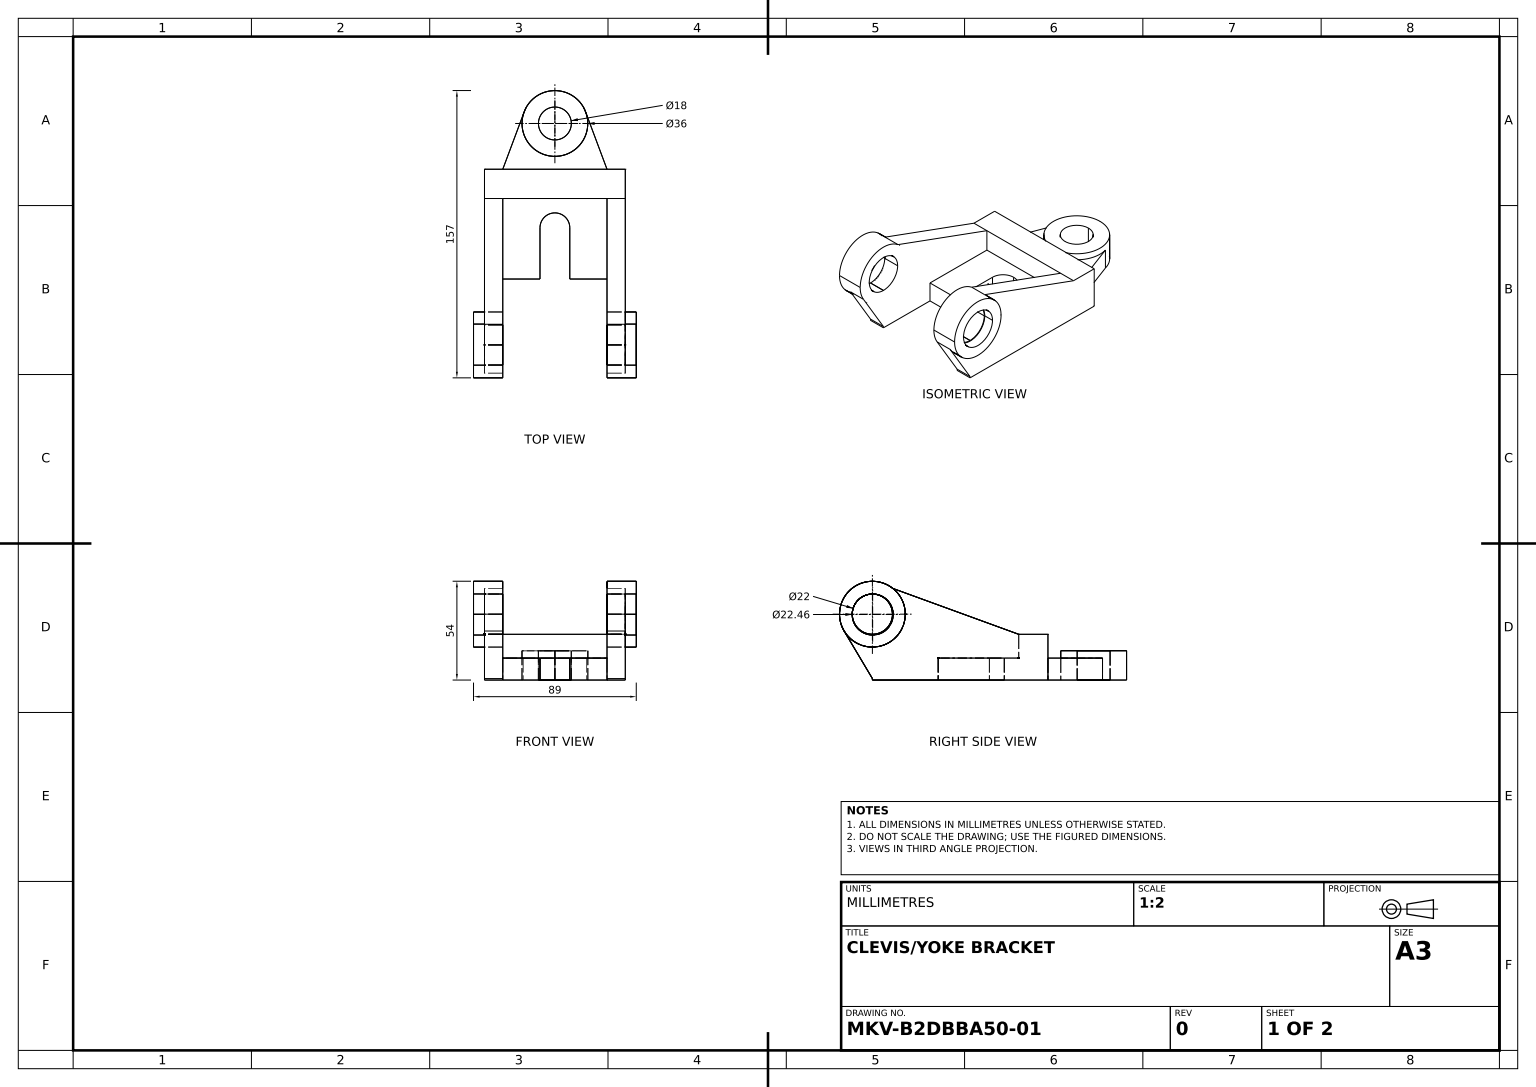
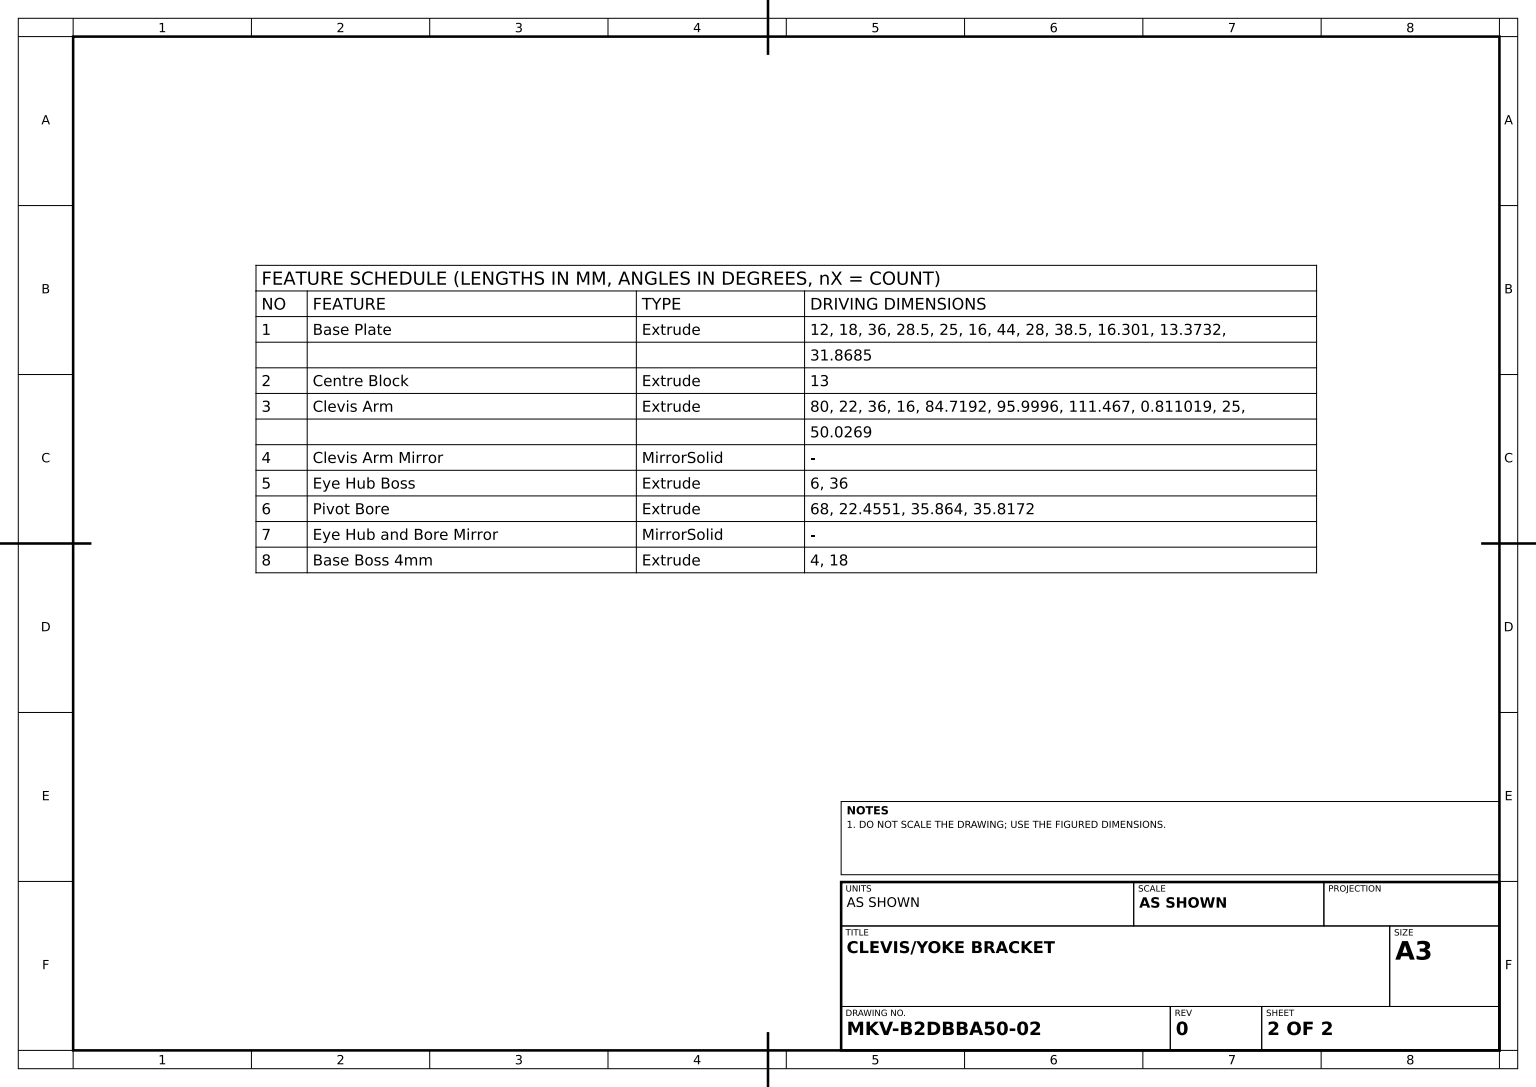
SolidWorks part; units mm, degrees
material "Plain Carbon Steel"
ref_plane "Front Plane" through (0, 0, 0) normal (0, 0, 1) x (1, 0, 0)
ref_plane "Top Plane" through (0, 0, 0) normal (0, 1, 0) x (1, 0, 0)
ref_plane "Right Plane" through (0, 0, 0) normal (1, 0, 0) x (0, 0, -1)
sketch "Base Plate Sketch" plane through (0, 0, 0) normal (0, 1, 0) x (1, 0, 0)
  line L0 (0, -13.3732) -> (-28.5, -13.3732)
  line L1 (-28.5, -13.3732) -> (28.5, -13.3732)
  line L2 (-28.5, -13.3732) -> (-17.3347, 16.4754)
  line L3 (17.3347, 16.4754) -> (28.5, -13.3732)
  line L4 (-8.1505, -45.3732) -> (-8.1505, -73.3732)
  line L5 (-28.5, -13.3732) -> (28.5, -13.3732)
  line L7 (-28.5, -29.3732) -> (28.5, -29.3732)
  line L9 (-28.5, -29.3732) -> (28.5, -29.3732)
  line L10 (-28.5, -29.3732) -> (-28.5, -73.3732)
  line L11 (-28.5, -73.3732) -> (-8.1505, -73.3732)
  line L12 (28.5, -29.3732) -> (28.5, -73.3732)
  line L13 (8.1505, -45.3732) -> (8.1505, -73.3732)
  line L14 (8.1505, -73.3732) -> (28.5, -73.3732)
  line L16 (-38.5, -13.3732) -> (38.5, -13.3732)
  line L17 (-38.5, -13.3732) -> (-38.5, -29.3732)
  line L18 (-38.5, -29.3732) -> (38.5, -29.3732)
  line L19 (38.5, -13.3732) -> (38.5, -29.3732)
  circle A0 centre (0, 11.6268) radius 9
  circle A1 centre (0, 11.6268) radius 18
  arc A2 (8.1505, -45.3732) -> (-8.1505, -45.3732) centre (0, -45.3732) ccw
  point P15 (0, -29.3732)
  dimension "D1" = 18
  dimension "D2" = 36
  dimension "D3" = 28.5
  dimension "D4" = 0
  dimension "D5" = 28.5
  dimension "D6" = 25
  dimension "D7" = 16
  dimension "D8" = 28.5
  dimension "D9" = 28.5
  dimension "D10" = 44
  dimension "D11" = 28
  dimension "D12" = 38.5
  dimension "D13" = 38.5
  dimension "D14" = 16.301
  dimension "D15" = 13.3732
  dimension "D16" = 31.8685
extrude "Base Plate" add sketch "Base Plate Sketch" along normal blind 12 contours A2 L13 L14 L12 L7 L10 L11 L4 | L19 L16 L1 L0 L17 L18 L7 | A1 L2 L0 L1 L3 | A1 A0
sketch "Centre Block Sketch" plane through (0, 12, 0) normal (0, 1, 0) x (1, 0, 0)
  line L1 (-38.5, -13.3732) -> (38.5, -13.3732)
  line L2 (-38.5, -13.3732) -> (-38.5, -29.3732)
  line L3 (-38.5, -29.3732) -> (38.5, -29.3732)
  line L4 (38.5, -13.3732) -> (38.5, -29.3732)
extrude "Centre Block" add sketch "Centre Block Sketch" along normal blind 13
sketch "Arm Reference Sketch" plane through (0, 0, 29.3732) normal (0, 0, 1) x (1, 0, 0)
  line L1 (38.5, 25) -> (28.5, 25)
  line L2 (38.5, 25) -> (38.5, 0)
  line L3 (38.5, 0) -> (28.5, 0)
  line L4 (28.5, 25) -> (28.5, 0)
  line L5 (-28.5, 0) -> (-38.5, 0)
  line L6 (-28.5, 0) -> (-28.5, 25)
  line L7 (-28.5, 25) -> (-38.5, 25)
  line L8 (-38.5, 0) -> (-38.5, 25)
sketch "Clevis Arm Sketch" plane through (38.5, 0, 0) normal (1, 0, 0) x (0, 0, -1)
  line L0 (-29.3732, 25) -> (-98.0924, 50.0269)
  line L1 (-29.3732, 0) -> (-109.3732, 0)
  line L2 (-29.3732, 0) -> (-29.3732, 25)
  line L3 (-109.3728, 25) -> (-109.3732, 25)
  line L4 (-109.3732, 0) -> (-109.3732, 0.811)
  line L5 (-109.3732, 0.811) -> (-124.8397, 26.7928)
  line L6 (-13.3732, 0) -> (-29.3732, 0) construction
  line L7 (-13.3732, 25) -> (-13.3732, 0) construction
  circle A0 centre (-109.3728, 36) radius 11
  circle A1 centre (-109.3728, 36) radius 18
  line M5 (-29.3732, 25) -> (-29.3732, 0)
  dimension "D2" = 22
  dimension "D3" = 36
  dimension "D1" = 80
  dimension "D4" = 36
  dimension "D5" = 16
  dimension "D6" = 84.7192
  dimension "D7" = 95.9996
  dimension "D8" = 111.4665
  dimension "D9" = 0.811
  dimension "D10" = 25
  dimension "D11" = 50.0269
extrude "Clevis Arm" add sketch "Clevis Arm Sketch" against normal up to vertex (10 mm away) contours A1 L5 L4 L1 L0 M5 | A1 A0 L3 up to point (28.5, 25, 29.3732)
mirror "Clevis Arm Mirror" about plane through (0, 0, 0) normal (1, 0, 0) of bodies 107
sketch "Eye Hub Sketch" plane through (38.5, 0, 0) normal (1, 0, 0) x (0, 0, -1)
  circle A0 centre (-109.3728, 36) radius 18
  dimension "D1" = 36
extrude "Eye Hub Boss" add sketch "Eye Hub Sketch" along normal blind 6
sketch "Pivot Bore Sketch" plane through (28.5, 0, 0) normal (-1, 0, 0) x (0, 0, 1)
  line L0 (73.3732, 12) -> (73.3732, 0) construction
  line L1 (73.3732, 0) -> (109.3732, 0) construction
  circle A0 centre (109.2372, 35.8172) radius 11.2275
  dimension "D1" = 22.4551
  dimension "D2" = 35.864
  dimension "D3" = 35.8172
extrude "Pivot Bore" cut sketch "Pivot Bore Sketch" against normal blind 68
mirror "Eye Hub and Bore Mirror" about plane through (0, 0, 0) normal (1, 0, 0) of bodies 110
sketch "Base Boss Sketch" plane through (0, 12, 0) normal (0, 1, 0) x (1, 0, 0)
  circle A0 centre (0, 11.6268) radius 18
  circle A1 centre (0, 11.6268) radius 9
  dimension "D1" = 18
extrude "Base Boss 4mm" add sketch "Base Boss Sketch" along normal blind 4
